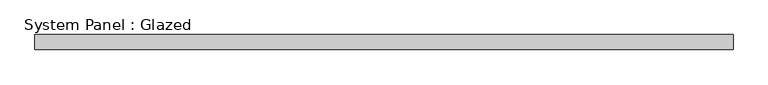
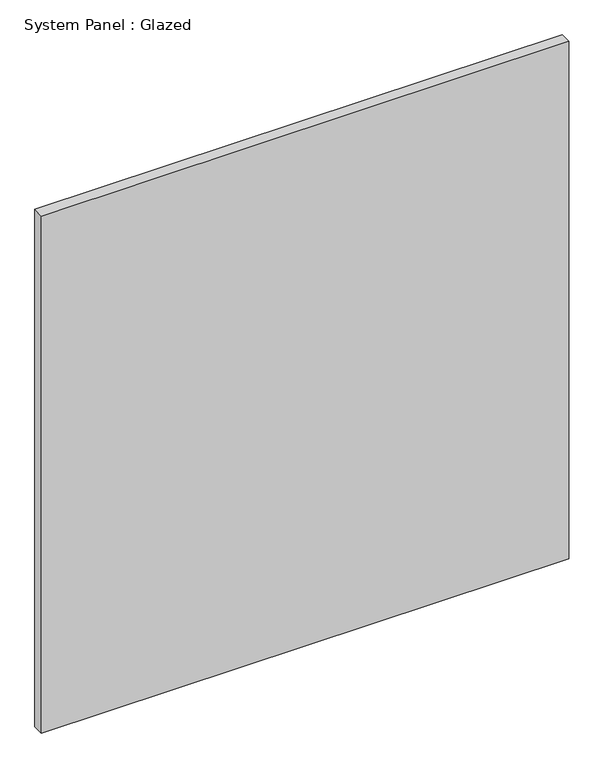
"""IFC4 building model written with IfcOpenShell, lengths in millimetres: plate geometry, System Panel : Glazed."""

from ifc_helpers import new_model, si_unit, origin, origin_with_axes, place, context, project, spatial, polyline, outline, extrude, source, transform, mapped, element, save


def system_panel_glazed_6dbe1261(model_context):
    return source(origin(), model_context, "Body", "SweptSolid", [
        extrude(outline(polyline([(587.8514963, 19.05), (-587.8514963, 19.05), (-587.8514963, 44.45), (587.8514963, 44.45), (587.8514963, 19.05)])), origin_with_axes(), (0.0, 0.0, 1.0), 1219.2),
    ])


if __name__ == "__main__":
    model = new_model("IFC4")
    model_context = context("Model", 3, world=origin())
    ifc_project = project(units=[si_unit("LENGTHUNIT", "METRE", prefix="MILLI")], contexts=[model_context])
    site = spatial("IfcSite", under=ifc_project)
    building = spatial("IfcBuilding", under=site)
    placement = place(None, origin())
    system_panel_glazed_shape = system_panel_glazed_6dbe1261(model_context)
    element("IfcPlate", 1, ObjectType="System Panel : Glazed", at=placement, inside=building, context=model_context, shape_type="MappedRepresentation", body=[
        mapped(system_panel_glazed_shape, transform((0.0, 0.0, 0.0), x_axis=(1.0, 0.0, 0.0), y_axis=(0.0, 1.0, 0.0), z_axis=(0.0, 0.0, 1.0))),
    ])
    save(model, "model.ifc")

# Revit data of these elements
# Type "System Panel : Glazed"
#   Construction Type Id = "GSP4R"
#   Analytic Construction = "1/8 in Pilkington single glazing"
#   Visual Light Transmittance = 0.9
#   Solar Heat Gain Coefficient = 0.86
#   Heat Transfer Coefficient (U) = 1.18115 BTU/(h·ft²·°F)
# Element 1 (IfcPlate, "System Panel : Glazed")
#   Materials on its faces: "Glass"
# Materials
#   "Glass": class "Glass", colour RGB 0 128 192, transparency 0.75, Description = "Soda Lime Glass", Cost = 0
